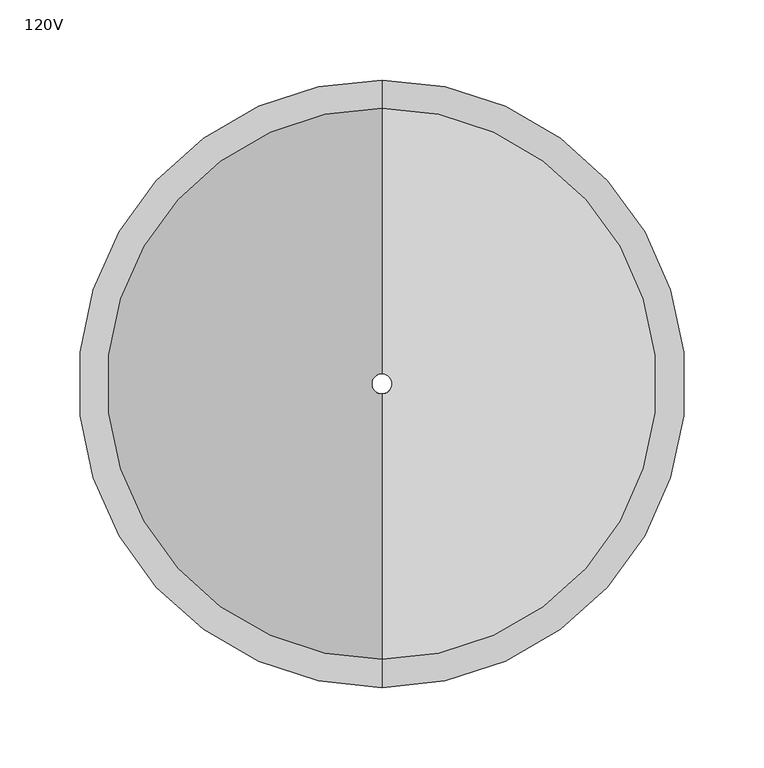
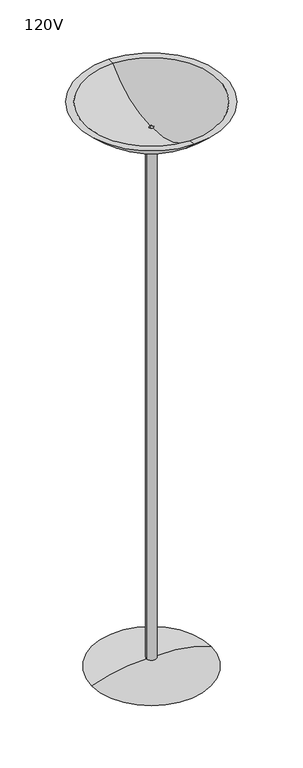
"""IFC4 building model written with IfcOpenShell, lengths in millimetres: light fixture geometry, 120V."""

from ifc_helpers import new_model, si_unit, point, frame, origin, place, context, project, spatial, polyline, circle_curve, ellipse_curve, trimmed, source, transform, mapped, element, save
from ifc_brep_helpers import plane_surface, cylinder_surface, revolved_surface, advanced_brep


def light_fixture_120v_8a54b260(model_context):
    return source(origin(), model_context, "Body", "AdvancedBrep", [
        advanced_brep(
        [(-12.7, 0.0, 23.8559377), (12.7, 0.0, 23.8559377), (152.4, 0.0, 0.0), (-152.4, 0.0, 0.0), (-12.7, 0.0, 1443.3755116), (12.7, 0.0, 1443.3755116), (-6.35, 0.0, 1443.3755116), (6.35, 0.0, 1443.3755116), (-6.35, 0.0, 0.0), (6.35, 0.0, 0.0)],
        [
            (0, 1, circle_curve(frame((0.0, 0.0, 23.8559377), z_axis=(0.0, 0.0, -1.0), x_axis=(0.0, 1.0, 0.0)), 12.7)),
            (1, 2, circle_curve(frame((27.9174306, 0.0, -307.9995076), z_axis=(0.0, 1.0, 0.0), x_axis=(1.0, 0.0, 0.0)), 332.2041643)),
            (2, 3, circle_curve(frame((0.0, 0.0, 0.0), z_axis=(0.0, 0.0, 1.0), x_axis=(0.0, 1.0, 0.0)), 152.4)),
            (3, 0, circle_curve(frame((-27.9174306, 0.0, -307.9995076), z_axis=(0.0, 1.0, 0.0), x_axis=(-1.0, 0.0, 0.0)), 332.2041643)),
            (1, 0, circle_curve(frame((0.0, 0.0, 23.8559377), z_axis=(0.0, 0.0, -1.0), x_axis=(0.0, 1.0, 0.0)), 12.7)),
            (3, 2, circle_curve(frame((0.0, 0.0, 0.0), z_axis=(0.0, 0.0, 1.0), x_axis=(0.0, 1.0, 0.0)), 152.4)),
            (4, 5, circle_curve(frame((0.0, 0.0, 1443.3755116), z_axis=(0.0, 0.0, -1.0), x_axis=(0.0, 1.0, 0.0)), 12.7)),
            (5, 1),
            (0, 4),
            (5, 4, circle_curve(frame((0.0, 0.0, 1443.3755116), z_axis=(0.0, 0.0, -1.0), x_axis=(0.0, 1.0, 0.0)), 12.7)),
            (6, 7, circle_curve(frame((0.0, 0.0, 1443.3755116), z_axis=(0.0, 0.0, -1.0), x_axis=(0.0, 1.0, 0.0)), 6.35)),
            (7, 5),
            (4, 6),
            (7, 6, circle_curve(frame((0.0, 0.0, 1443.3755116), z_axis=(0.0, 0.0, -1.0), x_axis=(0.0, 1.0, 0.0)), 6.35)),
            (8, 9, circle_curve(frame((0.0, 0.0, 0.0), z_axis=(0.0, 0.0, -1.0), x_axis=(0.0, 1.0, 0.0)), 6.35)),
            (9, 7),
            (6, 8),
            (9, 8, circle_curve(frame((0.0, 0.0, 0.0), z_axis=(0.0, 0.0, -1.0), x_axis=(0.0, 1.0, 0.0)), 6.35)),
            (2, 9),
            (8, 3),
        ],
        [
            revolved_surface(trimmed(ellipse_curve(frame((0.0, 27.9174306, -307.9995076), z_axis=(1.0, 0.0, 0.0), x_axis=(0.0, 1.0, 0.0)), 332.2041643, 332.2041643), [point((0.0, 152.4, 0.0))], [point((0.0, 12.7, 23.8559377))], True, "CARTESIAN"), (0.0, 0.0, 0.0), (0.0, 0.0, 1.0)),
            cylinder_surface(frame((0.0, 0.0, 0.0), z_axis=(0.0, 0.0, 1.0), x_axis=(0.0, 1.0, 0.0)), 12.7),
            plane_surface(frame((0.0, 0.0, 1443.3755116), z_axis=(0.0, 0.0, 1.0), x_axis=(0.0, 1.0, 0.0))),
            revolved_surface(polyline([(0.0, 6.35, 1443.3755116), (0.0, 6.35, 0.0)]), (0.0, 0.0, 0.0), (0.0, 0.0, 1.0)),
            plane_surface(frame((0.0, 0.0, 0.0), z_axis=(0.0, 0.0, -1.0), x_axis=(0.0, 1.0, 0.0))),
        ],
        [
            (0, [[1, 2, 3, 4]]),
            (0, [[5, -4, 6, -2]]),
            (1, [[7, 8, -1, 9]]),
            (1, [[10, -9, -5, -8]]),
            (2, [[11, 12, -7, 13]]),
            (2, [[14, -13, -10, -12]]),
            (3, [[15, 16, -11, 17]]),
            (3, [[18, -17, -14, -16]]),
            (4, [[-3, 19, -15, 20]]),
            (4, [[-6, -20, -18, -19]]),
        ],
    ),
        advanced_brep(
        [(0.0, -171.9151264, 1524.0), (0.0, 171.9151264, 1524.0), (0.0, 189.6566143, 1524.0), (0.0, -189.6566143, 1524.0), (0.0, -6.35, 1456.0755116), (0.0, 6.35, 1456.0755116), (0.0, -6.35, 1443.3755116), (0.0, 6.35, 1443.3755116), (0.0, -12.7, 1443.3755116), (0.0, 12.7, 1443.3755116)],
        [
            (0, 1, circle_curve(frame((0.0, 0.0, 1524.0), z_axis=(0.0, 0.0, -1.0), x_axis=(0.0, 1.0, 0.0)), 171.9151264)),
            (1, 2),
            (2, 3, circle_curve(frame((0.0, 0.0, 1524.0), z_axis=(0.0, 0.0, 1.0), x_axis=(0.0, 1.0, 0.0)), 189.6566143)),
            (3, 0),
            (1, 0, circle_curve(frame((0.0, 0.0, 1524.0), z_axis=(0.0, 0.0, -1.0), x_axis=(0.0, 1.0, 0.0)), 171.9151264)),
            (3, 2, circle_curve(frame((0.0, 0.0, 1524.0), z_axis=(0.0, 0.0, 1.0), x_axis=(0.0, 1.0, 0.0)), 189.6566143)),
            (4, 5, circle_curve(frame((0.0, 0.0, 1456.0755116), z_axis=(0.0, 0.0, -1.0), x_axis=(0.0, 1.0, 0.0)), 6.35)),
            (5, 1, circle_curve(frame((0.0, 6.35, 1691.8192616), z_axis=(1.0, 0.0, 0.0), x_axis=(0.0, 1.0, 0.0)), 235.74375)),
            (0, 4, circle_curve(frame((0.0, -6.35, 1691.8192616), z_axis=(1.0, 0.0, 0.0), x_axis=(0.0, -1.0, 0.0)), 235.74375)),
            (5, 4, circle_curve(frame((0.0, 0.0, 1456.0755116), z_axis=(0.0, 0.0, -1.0), x_axis=(0.0, 1.0, 0.0)), 6.35)),
            (6, 7, circle_curve(frame((0.0, 0.0, 1443.3755116), z_axis=(0.0, 0.0, -1.0), x_axis=(0.0, 1.0, 0.0)), 6.35)),
            (7, 5),
            (4, 6),
            (7, 6, circle_curve(frame((0.0, 0.0, 1443.3755116), z_axis=(0.0, 0.0, -1.0), x_axis=(0.0, 1.0, 0.0)), 6.35)),
            (8, 9, circle_curve(frame((0.0, 0.0, 1443.3755116), z_axis=(0.0, 0.0, -1.0), x_axis=(0.0, 1.0, 0.0)), 12.7)),
            (9, 7),
            (6, 8),
            (9, 8, circle_curve(frame((0.0, 0.0, 1443.3755116), z_axis=(0.0, 0.0, -1.0), x_axis=(0.0, 1.0, 0.0)), 12.7)),
            (2, 9, circle_curve(frame((0.0, 6.35, 1691.8192616), z_axis=(-1.0, 0.0, 0.0), x_axis=(0.0, 1.0, 0.0)), 248.5248869)),
            (8, 3, circle_curve(frame((0.0, -6.35, 1691.8192616), z_axis=(-1.0, 0.0, 0.0), x_axis=(0.0, -1.0, 0.0)), 248.5248869)),
        ],
        [
            plane_surface(frame((0.0, 0.0, 1524.0), z_axis=(0.0, 0.0, 1.0), x_axis=(0.0, 1.0, 0.0))),
            revolved_surface(trimmed(ellipse_curve(frame((0.0, 6.35, 1691.8192616), z_axis=(-1.0, 0.0, 0.0), x_axis=(0.0, 1.0, 0.0)), 235.74375, 235.74375), [point((0.0, 171.9151264, 1524.0))], [point((0.0, 6.35, 1456.0755116))], True, "CARTESIAN"), (0.0, 0.0, 1676.4), (0.0, 0.0, 1.0)),
            revolved_surface(polyline([(0.0, 6.35, 1456.0755116), (0.0, 6.35, 1443.3755116)]), (0.0, 0.0, 1676.4), (0.0, 0.0, 1.0)),
            plane_surface(frame((0.0, 0.0, 1443.3755116), z_axis=(0.0, 0.0, -1.0), x_axis=(0.0, 1.0, 0.0))),
            revolved_surface(trimmed(ellipse_curve(frame((0.0, 6.35, 1691.8192616), z_axis=(1.0, 0.0, 0.0), x_axis=(0.0, 1.0, 0.0)), 248.5248869, 248.5248869), [point((0.0, 12.7, 1443.3755116))], [point((0.0, 189.6566143, 1524.0))], True, "CARTESIAN"), (0.0, 0.0, 1676.4), (0.0, 0.0, 1.0)),
        ],
        [
            (0, [[1, 2, 3, 4]]),
            (0, [[5, -4, 6, -2]]),
            (1, [[7, 8, -1, 9]]),
            (1, [[10, -9, -5, -8]]),
            (2, [[11, 12, -7, 13]]),
            (2, [[14, -13, -10, -12]]),
            (3, [[15, 16, -11, 17]]),
            (3, [[18, -17, -14, -16]]),
            (4, [[-3, 19, -15, 20]]),
            (4, [[-6, -20, -18, -19]]),
        ],
    ),
    ])


if __name__ == "__main__":
    model = new_model("IFC4")
    model_context = context("Model", 3, world=origin())
    ifc_project = project(units=[si_unit("LENGTHUNIT", "METRE", prefix="MILLI")], contexts=[model_context])
    site = spatial("IfcSite", under=ifc_project)
    building = spatial("IfcBuilding", under=site)
    placement = place(None, origin())
    light_fixture_120v_shape = light_fixture_120v_8a54b260(model_context)
    element("IfcLightFixture", 1, ObjectType="120V", at=placement, inside=building, context=model_context, shape_type="MappedRepresentation", body=[
        mapped(light_fixture_120v_shape, transform((0.0, 0.0, 0.0), x_axis=(1.0, 0.0, 0.0), y_axis=(0.0, 1.0, 0.0), z_axis=(0.0, 0.0, 1.0))),
    ])
    save(model, "model.ifc")

# Revit data of these elements
# Type "120V"
#   Wattage Comments = "100"
#   Lamp = "T-4"
#   Assembly Code = "D5020230"
#   Wattage = 100 W
#   built-in parameter 1150110 = 1 (stored number, unit not read)
#   built-in parameter 1114217 = 1 (stored number, unit not read)
#   built-in parameter 1150109 = 1 (stored number, unit not read)
#   built-in parameter 1150113 = 1 (stored number, unit not read)
#   Lumens = 1800 lm
#   built-in parameter 1150115 = 1 (stored number, unit not read)
#   built-in parameter 1150105 = 572.958 (stored number, unit not read)
#   Light Source Symbol Size = 2' - 0"
#   built-in parameter 1150112 = 1 (stored number, unit not read)
#   built-in parameter 1150114 = 1 (stored number, unit not read)
#   built-in parameter 1150107 = 3200 (stored number, unit not read)
#   built-in parameter 1150106 = 5.72958 (stored number, unit not read)
#   Height = 5' - 0"
#   built-in parameter 1150104 = 1.67225 (stored number, unit not read)
#   Ballast Voltage = 120 V
#   built-in parameter 1114218 = 1 (stored number, unit not read)
#   built-in parameter 1150133 = 10 (stored number, unit not read)
#   Apparent Load = 100 VA
#   built-in parameter 1150134 = 3
#   built-in parameter 1150137 = 1
#   Color Filter = 16777215
#   Ballast Number of Poles = 1
#   Shade = Glass, Frosted
#   Stand = Steel, Chrome Plated
#   Dimming Lamp Color Temperature Shift = (empty or 0)
#   Default Elevation = 0
# Element 1 (IfcLightFixture, "120V")
#   Materials on its faces: "Steel, Chrome Plated", "Glass, Frosted"
# Materials
#   "Glass, Frosted": class "Glass", colour RGB 250 244 225, transparency 0.55, Description = "physical material", Cost = 0
#   "Steel, Chrome Plated": class "Metal", colour RGB 17 17 17, transparency 0, Description = "Chromiuim plated steel", Cost = 0
